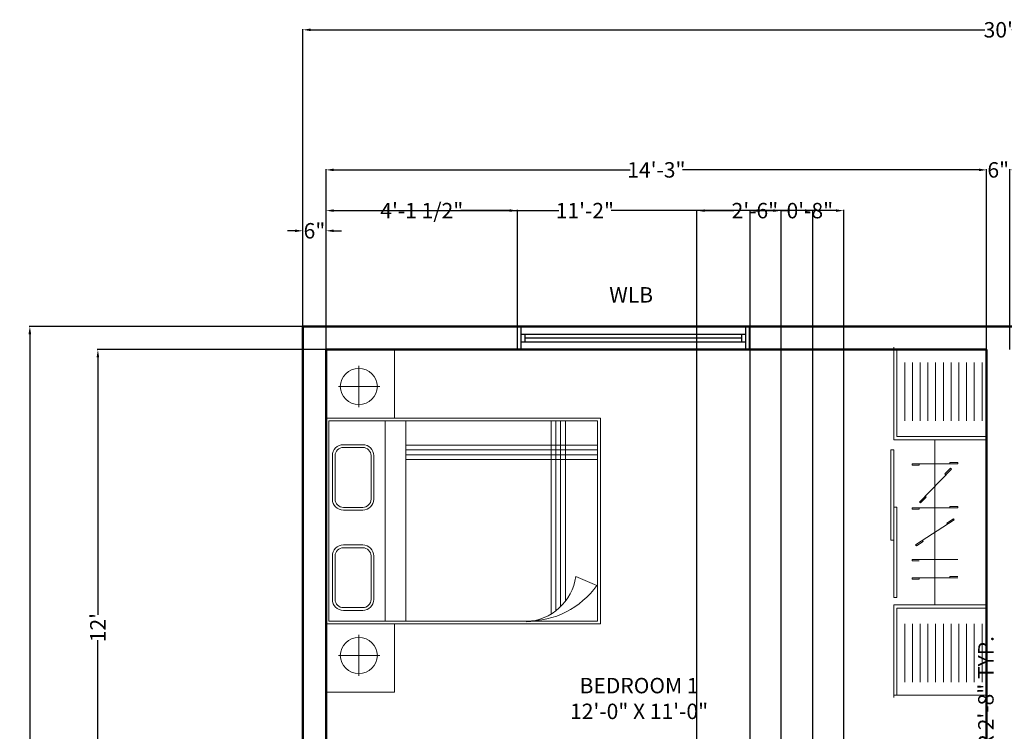
# Model space of a CAD drawing. Units: inches. Extents: x 2663 to 3147, y 140 to 736.
# Tile 5 of 6: x 2663 to 2918, y 551 to 736. Entities that reach past the tile are written whole.
import ezdxf

# ---------------------------------------------------------------- set-up
doc = ezdxf.new("R2010")
doc.units = ezdxf.units.IN
doc.header["$MEASUREMENT"] = 0
for name, color, linetype, lineweight in [('A-ANNO-DIMS', 2, 'Continuous', 18), ('A-AREA-IDEN', 3, 'Continuous', 25), ('A-FURN', 8, 'Continuous', 18), ('A-GLAZ', 4, 'Continuous', 25), ('A-WALL', 7, 'Continuous', 50)]:
    doc.layers.add(name, color=color, linetype=linetype, lineweight=lineweight)
doc.styles.get("Standard").update_dxf_attribs({"font": 'arial.ttf'})
doc.dimstyles.get("Standard").update_dxf_attribs({"dimtxt": 4, "dimasz": 2, "dimexe": 0.18, "dimexo": 0.0625, "dimgap": 0.09, "dimtad": 0, "dimdec": 0, "dimzin": 0, "dimdsep": 46, "dimlunit": 4, "dimtxsty": 'Standard', "dimcen": 0.09, "dimadec": 0, "dimazin": 0, "dimtfac": 1, "dimtdec": 0, "dimtofl": 0, "dimtmove": 0, "dimatfit": 3, "dimfxl": 1, "dimtolj": 1, "dimtzin": 0, "dimarcsym": 0})

# ---------------------------------------------------------------- blocks, each defined once
blk = doc.blocks.new('*D1')
at = {"layer": 'A-ANNO-DIMS', "color": 0, "lineweight": -2, "transparency": 16777216}
for p, q in [((2742.16, 650.39), (2742.16, 697.05)), ((2744.16, 696.87), (2820.89, 696.87)), ((2911.16, 696.87), (2834.43, 696.87)), ((2913.16, 650.39), (2913.16, 697.05))]:
    blk.add_line(p, q, dxfattribs=at)
at = {"layer": 'A-ANNO-DIMS', "color": 0, "transparency": 16777216}
for points in [[(2744.16, 697.21), (2744.16, 696.54), (2742.16, 696.87)], [(2911.16, 697.21), (2911.16, 696.54), (2913.16, 696.87)]]:
    blk.add_solid(points, dxfattribs=at)
at = {"layer": 'Defpoints', "color": 0, "transparency": 16777216}
for p in [(2913.16, 696.87), (2742.16, 650.32), (2913.16, 650.32)]:
    blk.add_point(p, dxfattribs=at)
at = {"layer": 'A-ANNO-DIMS', "color": 0, "transparency": 16777216, "insert": (2827.66, 696.87), "char_height": 4, "attachment_point": 5}
blk.add_mtext('\\A1;14\'-3"', dxfattribs=at)
blk = doc.blocks.new('*D2')
at = {"layer": 'A-ANNO-DIMS', "color": 0, "lineweight": -2, "transparency": 16777216}
for p, q in [((2911.16, 696.87), (2909.16, 696.87)), ((2913.16, 650.39), (2913.16, 697.05)), ((2919.16, 650.39), (2919.16, 697.05)), ((2921.16, 696.87), (2923.16, 696.87))]:
    blk.add_line(p, q, dxfattribs=at)
at = {"layer": 'A-ANNO-DIMS', "color": 0, "transparency": 16777216}
for points in [[(2911.16, 697.21), (2911.16, 696.54), (2913.16, 696.87)], [(2921.16, 697.21), (2921.16, 696.54), (2919.16, 696.87)]]:
    blk.add_solid(points, dxfattribs=at)
at = {"layer": 'Defpoints', "color": 0, "transparency": 16777216}
for p in [(2919.16, 696.87), (2913.16, 650.32), (2919.16, 650.32)]:
    blk.add_point(p, dxfattribs=at)
at = {"layer": 'A-ANNO-DIMS', "color": 0, "transparency": 16777216, "insert": (2916.16, 696.87), "char_height": 4, "attachment_point": 5}
blk.add_mtext('\\A1;6"', dxfattribs=at)
blk = doc.blocks.new('EDFRTYUI')
for p, q in [((3325.9, 253.54), (3325.9, 259.54)), ((3325.9, 259.54), (3385.9, 259.54)), ((3326.9, 253.54), (3326.9, 259.54)), ((3326.9, 257.54), (3384.9, 257.54)), ((3327.9, 255.54), (3327.9, 257.54)), ((3383.9, 257.54), (3383.9, 255.54)), ((3384.9, 259.54), (3384.9, 253.54)), ((3385.9, 259.54), (3385.9, 253.54)), ((3326.9, 255.54), (3384.9, 255.54)), ((3327.9, 256.54), (3383.9, 256.54)), ((3385.9, 253.54), (3325.9, 253.54))]:
    blk.add_line(p, q)
at = {"insert": (3337.87, 269.72), "char_height": 4, "attachment_point": 1}
blk.add_mtext_dynamic_manual_height_columns('\\pxqc;WLB', width=34.9199, gutter_width=20, heights=[0], dxfattribs=at)
blk = doc.blocks.new('A$C34930FF8')
at = {"ltscale": 0.05}
for p, q in [((0, 2252.4), (0, 16.8)), ((600, 2252.4), (0, 2252.4)), ((185.4, 1513), (185.4, 1521.5)), ((227.1, 1479.2), (233.2, 1485.2)), ((237.7, 1513), (237.7, 1521.5)), ((436.7, 1513), (436.7, 1504.4)), ((482.5, 1513), (482.5, 1504.4)), ((263.6, 1441.7), (269.7, 1447.7)), ((398.2, 1303.6), (392.1, 1297.6)), ((185.4, 1229.1), (185.4, 1237.7)), ((237.7, 1229.1), (237.7, 1237.7)), ((434.8, 1266.1), (428.7, 1260.1)), ((436.7, 1228.2), (436.7, 1219.7)), ((482.5, 1228.2), (482.5, 1219.7)), ((209.5, 1150.1), (214.1, 1157.3)), ((253.5, 1121.8), (258.1, 1129)), ((415.3, 1017.6), (410.6, 1010.5)), ((459.3, 989.3), (454.7, 982.1)), ((482.5, 894.9), (482.5, 886.3)), ((237.7, 775.3), (237.7, 783.9)), ((436.7, 775.3), (436.7, 766.8)), ((482.5, 775.3), (482.5, 766.8)), ((600, 16.8), (0, 16.8))]:
    blk.add_line(p, q, dxfattribs=at)
for p, q in [((580, 1690.9), (580, 2252.4)), ((600, 1669.3), (600, 2269.3)), ((30, 1790.9), (30, 2169.3)), ((80, 1790.9), (80, 2169.3)), ((130, 1790.9), (130, 2169.3)), ((180, 1790.9), (180, 2169.3)), ((230, 1790.9), (230, 2169.3)), ((280, 1790.9), (280, 2169.3)), ((330, 1790.9), (330, 2169.3)), ((380, 1790.9), (380, 2169.3)), ((430, 1790.9), (430, 2169.3)), ((480, 1790.9), (480, 2169.3)), ((530, 1790.9), (530, 2169.3)), ((580, 1690.9), (0, 1690.9)), ((600, 1669.3), (0, 1669.3)), ((335.4, 1666.1), (335.4, 603.1)), ((600, 1603.3), (620, 1603.3)), ((600, 1018.7), (600, 1603.3)), ((620, 1603.3), (620, 1018.7)), ((237.7, 1521.5), (185.4, 1521.5)), ((482.5, 1513), (185.4, 1513)), ((434.8, 1266.1), (227.4, 1478.9)), ((269.7, 1447.7), (233.2, 1485.2)), ((436.7, 1504.4), (482.5, 1504.4)), ((428.7, 1260.1), (392.1, 1297.6)), ((237.7, 1237.7), (185.4, 1237.7)), ((482.5, 1228.2), (185.4, 1228.2)), ((436.7, 1219.7), (482.5, 1219.7)), ((600, 1233.4), (580, 1233.4)), ((580, 1233.4), (580, 648.7)), ((600, 648.7), (600, 1233.4)), ((459.3, 989.3), (209.5, 1150.1)), ((258.1, 1129), (214.1, 1157.3)), ((454.7, 982.1), (410.6, 1010.5)), ((620, 1018.7), (600, 1018.7)), ((482.5, 894.9), (185.4, 894.9)), ((436.7, 886.3), (482.5, 886.3)), ((237.7, 783.9), (185.4, 783.9)), ((482.5, 775.3), (185.4, 775.3)), ((436.7, 766.8), (482.5, 766.8)), ((580, 648.7), (600, 648.7)), ((600, 600), (0, 600)), ((580, 578.3), (0, 578.3)), ((580, 578.3), (580, 16.8)), ((600, 600), (600, 0)), ((30, 478.3), (30, 100)), ((80, 478.3), (80, 100)), ((130, 478.3), (130, 100)), ((180, 478.3), (180, 100)), ((230, 478.3), (230, 100)), ((280, 478.3), (280, 100)), ((330, 478.3), (330, 100)), ((380, 478.3), (380, 100)), ((430, 478.3), (430, 100)), ((480, 478.3), (480, 100)), ((530, 478.3), (530, 100))]:
    blk.add_line(p, q)
blk = doc.blocks.new('A$C057D194F')
for p, q in [((0, 1.5, -0.1688), (0, 2, -0.1688)), ((0, 2, -0.1688), (0.5, 2, -0.1688)), ((0.5, 2, -0.1688), (0.5, 0, -0.1688)), ((2, 2, -0.1688), (0.5, 2, -0.1688)), ((1.98, 1.98, -0.1688), (0.52, 1.98, -0.1688)), ((0.52, 1.98, -0.1688), (0.52, 0.02, -0.1688)), ((1.0907, 1.9539, -0.1688), (0.7735, 1.9539, -0.1688)), ((1.8224, 1.9539, -0.1688), (1.5052, 1.9539, -0.1688)), ((1.98, 0.02, -0.1688), (1.98, 1.98, -0.1688)), ((2, 0, -0.1688), (2, 2, -0.1688)), ((2.5, 2, -0.1688), (2, 2, -0.1688)), ((2.5, 1.5, -0.1688), (2.5, 2, -0.1688)), ((0.2687, 1.9081, -0.1688), (0.2687, 1.761, -0.1688)), ((0.2687, 1.6081, -0.1688), (0.2687, 1.9081, -0.1688)), ((0.6935, 1.8739, -0.1688), (0.6935, 1.7322, -0.1688)), ((0.7135, 1.8739, -0.1688), (0.7135, 1.7322, -0.1688)), ((1.0907, 1.9339, -0.1688), (0.7735, 1.9339, -0.1688)), ((1.1507, 1.7322, -0.1688), (1.1507, 1.8739, -0.1688)), ((1.1707, 1.7322, -0.1688), (1.1707, 1.8739, -0.1688)), ((1.4252, 1.8739, -0.1688), (1.4252, 1.7322, -0.1688)), ((1.4452, 1.8739, -0.1688), (1.4452, 1.7322, -0.1688)), ((1.8224, 1.9339, -0.1688), (1.5052, 1.9339, -0.1688)), ((1.8824, 1.7322, -0.1688), (1.8824, 1.8739, -0.1688)), ((1.9024, 1.7322, -0.1688), (1.9024, 1.8739, -0.1688)), ((2.2313, 1.9081, -0.1688), (2.2313, 1.761, -0.1688)), ((2.2313, 1.6081, -0.1688), (2.2313, 1.9081, -0.1688)), ((0.4194, 1.761, -0.1688), (0.1194, 1.761, -0.1688)), ((0.2687, 1.761, -0.1688), (0.4194, 1.761, -0.1688)), ((0.2687, 1.761, -0.1688), (0.2687, 1.6081, -0.1688)), ((2.0806, 1.761, -0.1688), (2.3806, 1.761, -0.1688)), ((2.2313, 1.761, -0.1688), (2.0806, 1.761, -0.1688)), ((2.2313, 1.761, -0.1688), (2.2313, 1.6081, -0.1688)), ((0.7735, 1.6722, -0.1688), (1.0907, 1.6722, -0.1688)), ((0.7735, 1.6522, -0.1688), (1.0907, 1.6522, -0.1688)), ((1.5052, 1.6722, -0.1688), (1.8224, 1.6722, -0.1688)), ((1.5052, 1.6522, -0.1688), (1.8224, 1.6522, -0.1688)), ((1.98, 1.5693, -0.1688), (0.52, 1.5693, -0.1688)), ((0.5, 1.5, -0.1688), (0, 1.5, -0.1688)), ((2, 1.5, -0.1688), (2.5, 1.5, -0.1688)), ((1.98, 1.4193, -0.1688), (0.52, 1.4193, -0.1688)), ((0.6969, 0.02, -0.1688), (0.6969, 1.4193, -0.1688)), ((0.7319, 0.02, -0.1688), (0.7319, 1.4193, -0.1688)), ((0.7669, 0.02, -0.1688), (0.7669, 1.4193, -0.1688)), ((0.8019, 0.02, -0.1688), (0.8019, 1.4193, -0.1688)), ((0.52, 0.3595, -0.1688), (1.9292, 0.3595, -0.1688)), ((0.52, 0.3245, -0.1688), (1.905, 0.3245, -0.1688)), ((0.52, 0.2895, -0.1688), (1.8742, 0.2895, -0.1688)), ((0.52, 0.2545, -0.1688), (1.8344, 0.2545, -0.1688)), ((1.6548, 0.1789, -0.1688), (1.7198, 0.0251, -0.1688)), ((0.52, 0.02, -0.1688), (1.98, 0.02, -0.1688)), ((0.5, 0, -0.1688), (2, 0, -0.1688))]:
    blk.add_line(p, q)
for centre, radius, start, end in [((0.7735, 1.8739, -0.1688), 0.08, 90, 180), ((1.0907, 1.8739, -0.1688), 0.08, 0, 90), ((1.5052, 1.8739, -0.1688), 0.08, 90, 180), ((1.8224, 1.8739, -0.1688), 0.08, 0, 90), ((0.7735, 1.8739, -0.1688), 0.06, 90, 180), ((1.0907, 1.8739, -0.1688), 0.06, 0, 90), ((1.5052, 1.8739, -0.1688), 0.06, 90, 180), ((1.8224, 1.8739, -0.1688), 0.06, 0, 90), ((0.7735, 1.7322, -0.1688), 0.08, 180, 270), ((0.7735, 1.7322, -0.1688), 0.06, 180, 270), ((1.0907, 1.7322, -0.1688), 0.08, 270, 0), ((1.0907, 1.7322, -0.1688), 0.06, 270, 0), ((1.5052, 1.7322, -0.1688), 0.08, 180, 270), ((1.5052, 1.7322, -0.1688), 0.06, 180, 270), ((1.8224, 1.7322, -0.1688), 0.08, 270, 0), ((1.8224, 1.7322, -0.1688), 0.06, 270, 0), ((1.5992, 0.5623, -0.1688), 0.3874, 278.2518, 356.6808), ((1.363, 0.5286, -0.1688), 0.6171, 305.32946, 1.04595)]:
    blk.add_arc(centre, radius, start, end)
blk.add_ellipse((0.2687, 1.761, -0.1688), major_axis=(0, -0.1351), ratio=0.975448)
at = {"extrusion": (0, 0, -1)}
blk.add_ellipse((2.2313, 1.761, -0.1688), major_axis=(0, 0.1351), ratio=0.975448, dxfattribs=at)
for p in [(0.2687, 1.761, -0.1688), (2.2313, 1.761, -0.1688)]:
    blk.add_point(p)
blk = doc.blocks.new('*D21')
at = {"layer": 'A-ANNO-DIMS', "color": 0, "lineweight": -2, "transparency": 16777216}
for p, q in [((2734.16, 681.1), (2732.16, 681.1)), ((2736.16, 656.39), (2736.16, 681.28)), ((2742.16, 650.39), (2742.16, 681.28)), ((2744.16, 681.1), (2746.16, 681.1))]:
    blk.add_line(p, q, dxfattribs=at)
at = {"layer": 'A-ANNO-DIMS', "color": 0, "transparency": 16777216}
for points in [[(2734.16, 681.43), (2734.16, 680.76), (2736.16, 681.1)], [(2744.16, 681.43), (2744.16, 680.76), (2742.16, 681.1)]]:
    blk.add_solid(points, dxfattribs=at)
at = {"layer": 'Defpoints', "color": 0, "transparency": 16777216}
for p in [(2742.16, 681.1), (2736.16, 656.32), (2742.16, 650.32)]:
    blk.add_point(p, dxfattribs=at)
at = {"layer": 'A-ANNO-DIMS', "color": 0, "transparency": 16777216, "insert": (2739.16, 681.1), "char_height": 4, "attachment_point": 5}
blk.add_mtext('\\A1;6"', dxfattribs=at)
blk = doc.blocks.new('*D36')
at = {"layer": 'A-ANNO-DIMS', "color": 0, "lineweight": -2, "transparency": 16777216}
for p, q in [((2742.1, 650.32), (2682.92, 650.32)), ((2683.1, 648.32), (2683.1, 581.62)), ((2683.1, 508.32), (2683.1, 575.03)), ((2742.1, 506.32), (2682.92, 506.32))]:
    blk.add_line(p, q, dxfattribs=at)
at = {"layer": 'A-ANNO-DIMS', "color": 0, "transparency": 16777216}
for points in [[(2682.77, 648.32), (2683.44, 648.32), (2683.1, 650.32)], [(2682.77, 508.32), (2683.44, 508.32), (2683.1, 506.32)]]:
    blk.add_solid(points, dxfattribs=at)
at = {"layer": 'Defpoints', "color": 0, "transparency": 16777216}
for p in [(2683.1, 650.32), (2742.16, 650.32), (2742.16, 506.32)]:
    blk.add_point(p, dxfattribs=at)
at = {"layer": 'A-ANNO-DIMS', "color": 0, "transparency": 16777216, "insert": (2683.1, 578.32), "char_height": 4, "attachment_point": 5, "rotation": 90}
blk.add_mtext("\\A1;12'", dxfattribs=at)
blk = doc.blocks.new('*D37')
at = {"layer": 'A-ANNO-DIMS', "color": 0, "lineweight": -2, "transparency": 16777216}
for p, q in [((2736.1, 656.32), (2665.31, 656.32)), ((2665.49, 654.32), (2665.49, 419.89)), ((2665.49, 178.32), (2665.49, 412.76)), ((2736.1, 176.32), (2665.31, 176.32))]:
    blk.add_line(p, q, dxfattribs=at)
at = {"layer": 'A-ANNO-DIMS', "color": 0, "transparency": 16777216}
for points in [[(2665.15, 654.32), (2665.82, 654.32), (2665.49, 656.32)], [(2665.15, 178.32), (2665.82, 178.32), (2665.49, 176.32)]]:
    blk.add_solid(points, dxfattribs=at)
at = {"layer": 'Defpoints', "color": 0, "transparency": 16777216}
for p in [(2665.49, 656.32), (2736.16, 656.32), (2736.16, 176.32)]:
    blk.add_point(p, dxfattribs=at)
at = {"layer": 'A-ANNO-DIMS', "color": 0, "transparency": 16777216, "insert": (2665.49, 416.32), "char_height": 4, "attachment_point": 5, "rotation": 90}
blk.add_mtext("\\A1;40'", dxfattribs=at)
blk = doc.blocks.new('*D38')
at = {"layer": 'A-ANNO-DIMS', "color": 0, "lineweight": -2, "transparency": 16777216}
for p, q in [((2736.16, 656.39), (2736.16, 733.33)), ((2738.16, 733.15), (2912.68, 733.15)), ((3094.16, 733.15), (2919.64, 733.15)), ((3096.16, 656.39), (3096.16, 733.33))]:
    blk.add_line(p, q, dxfattribs=at)
at = {"layer": 'A-ANNO-DIMS', "color": 0, "transparency": 16777216}
for points in [[(2738.16, 733.48), (2738.16, 732.82), (2736.16, 733.15)], [(3094.16, 733.48), (3094.16, 732.82), (3096.16, 733.15)]]:
    blk.add_solid(points, dxfattribs=at)
at = {"layer": 'Defpoints', "color": 0, "transparency": 16777216}
for p in [(3096.16, 733.15), (2736.16, 656.32), (3096.16, 656.32)]:
    blk.add_point(p, dxfattribs=at)
at = {"layer": 'A-ANNO-DIMS', "color": 0, "transparency": 16777216, "insert": (2916.16, 733.15), "char_height": 4, "attachment_point": 5}
blk.add_mtext("\\A1;30'", dxfattribs=at)
blk = doc.blocks.new('*D39')
at = {"layer": 'A-ANNO-DIMS', "color": 0, "lineweight": -2, "transparency": 16777216}
for p, q in [((2912.96, 532.32), (2912.96, 534.32)), ((2908.22, 532.32), (2913.14, 532.32)), ((2912.96, 502.32), (2912.96, 530.32)), ((2908.22, 500.32), (2913.14, 500.32))]:
    blk.add_line(p, q, dxfattribs=at)
at = {"layer": 'A-ANNO-DIMS', "color": 0, "transparency": 16777216}
for points in [[(2912.63, 530.32), (2913.29, 530.32), (2912.96, 532.32)], [(2912.63, 502.32), (2913.29, 502.32), (2912.96, 500.32)]]:
    blk.add_solid(points, dxfattribs=at)
at = {"layer": 'Defpoints', "color": 0, "transparency": 16777216}
for p in [(2908.16, 532.32), (2912.96, 532.32), (2908.16, 500.32)]:
    blk.add_point(p, dxfattribs=at)
at = {"layer": 'A-ANNO-DIMS', "color": 0, "transparency": 16777216, "insert": (2912.96, 555.66), "char_height": 4, "attachment_point": 5, "rotation": 90}
blk.add_mtext('\\A1;DOOR 2\'-8" TYP.', dxfattribs=at)
blk = doc.blocks.new('*D61')
at = {"layer": 'A-ANNO-DIMS', "color": 0, "lineweight": -2, "transparency": 16777216}
for p, q in [((2851.95, 276.84), (2851.95, 686.5)), ((2853.95, 686.32), (2857.98, 686.32)), ((2859.98, 276.84), (2859.98, 686.5)), ((2859.98, 686.32), (2861.98, 686.32))]:
    blk.add_line(p, q, dxfattribs=at)
at = {"layer": 'A-ANNO-DIMS', "color": 0, "transparency": 16777216}
for points in [[(2853.95, 686.66), (2853.95, 685.99), (2851.95, 686.32)], [(2857.98, 686.66), (2857.98, 685.99), (2859.98, 686.32)]]:
    blk.add_solid(points, dxfattribs=at)
at = {"layer": 'Defpoints', "color": 0, "transparency": 16777216}
for p in [(2859.98, 686.32), (2851.95, 276.78), (2859.98, 276.78)]:
    blk.add_point(p, dxfattribs=at)
at = {"layer": 'A-ANNO-DIMS', "color": 0, "transparency": 16777216, "insert": (2867.39, 686.32), "char_height": 4, "attachment_point": 5}
blk.add_mtext('\\A1;0\'-8"', dxfattribs=at)
blk = doc.blocks.new('*D68')
at = {"layer": 'A-ANNO-DIMS', "color": 0, "lineweight": -2, "transparency": 16777216}
for p, q in [((2742.16, 650.39), (2742.16, 686.5)), ((2744.16, 686.32), (2756.79, 686.32)), ((2789.71, 686.32), (2777.08, 686.32)), ((2791.71, 650.39), (2791.71, 686.5))]:
    blk.add_line(p, q, dxfattribs=at)
at = {"layer": 'A-ANNO-DIMS', "color": 0, "transparency": 16777216}
for points in [[(2744.16, 686.66), (2744.16, 685.99), (2742.16, 686.32)], [(2789.71, 686.66), (2789.71, 685.99), (2791.71, 686.32)]]:
    blk.add_solid(points, dxfattribs=at)
at = {"layer": 'Defpoints', "color": 0, "transparency": 16777216}
for p in [(2791.71, 686.32), (2742.16, 650.32), (2791.71, 650.32)]:
    blk.add_point(p, dxfattribs=at)
at = {"layer": 'A-ANNO-DIMS', "color": 0, "transparency": 16777216, "insert": (2766.94, 686.32), "char_height": 4, "attachment_point": 5}
blk.add_mtext('\\A1;4\'-1 1/2"', dxfattribs=at)
blk = doc.blocks.new('*D75')
at = {"layer": 'A-ANNO-DIMS', "color": 0, "lineweight": -2, "transparency": 16777216}
for p, q in [((2742.16, 506.39), (2742.16, 686.5)), ((2744.16, 686.32), (2802.39, 686.32)), ((2874.16, 686.32), (2815.93, 686.32)), ((2876.16, 506.39), (2876.16, 686.5))]:
    blk.add_line(p, q, dxfattribs=at)
at = {"layer": 'A-ANNO-DIMS', "color": 0, "transparency": 16777216}
for points in [[(2744.16, 686.66), (2744.16, 685.99), (2742.16, 686.32)], [(2874.16, 686.66), (2874.16, 685.99), (2876.16, 686.32)]]:
    blk.add_solid(points, dxfattribs=at)
at = {"layer": 'Defpoints', "color": 0, "transparency": 16777216}
for p in [(2876.16, 686.32), (2742.16, 506.32), (2876.16, 506.32)]:
    blk.add_point(p, dxfattribs=at)
at = {"layer": 'A-ANNO-DIMS', "color": 0, "transparency": 16777216, "insert": (2809.16, 686.32), "char_height": 4, "attachment_point": 5}
blk.add_mtext('\\A1;11\'-2"', dxfattribs=at)
blk = doc.blocks.new('*D78')
at = {"layer": 'A-ANNO-DIMS', "color": 0, "lineweight": -2, "transparency": 16777216}
for p, q in [((2838.16, 440.39), (2838.16, 686.5)), ((2840.16, 686.32), (2847.72, 686.32)), ((2866.16, 686.32), (2858.6, 686.32)), ((2868.16, 440.39), (2868.16, 686.5))]:
    blk.add_line(p, q, dxfattribs=at)
at = {"layer": 'A-ANNO-DIMS', "color": 0, "transparency": 16777216}
for points in [[(2840.16, 686.66), (2840.16, 685.99), (2838.16, 686.32)], [(2866.16, 686.66), (2866.16, 685.99), (2868.16, 686.32)]]:
    blk.add_solid(points, dxfattribs=at)
at = {"layer": 'Defpoints', "color": 0, "transparency": 16777216}
for p in [(2868.16, 686.32), (2838.16, 440.32), (2868.16, 440.32)]:
    blk.add_point(p, dxfattribs=at)
at = {"layer": 'A-ANNO-DIMS', "color": 0, "transparency": 16777216, "insert": (2853.16, 686.32), "char_height": 4, "attachment_point": 5}
blk.add_mtext('\\A1;2\'-6"', dxfattribs=at)

msp = doc.modelspace()

# ---------------------------------------------------------------- linework, layer by layer
at = {"layer": 'A-WALL'}
for p, q in [((2736.16, 656.32), (3096.16, 656.32)), ((2736.16, 176.32), (2736.16, 656.32)), ((2742.16, 650.32), (2913.16, 650.32)), ((2742.16, 506.32), (2742.16, 650.32)), ((2913.16, 650.32), (2913.16, 506.32))]:
    msp.add_line(p, q, dxfattribs=at)

# ---------------------------------------------------------------- block references
at = {"layer": 'A-FURN', "xscale": -35.50398587953096, "yscale": 35.50398587953096, "zscale": 35.50398587953096, "rotation": 90}
msp.add_blockref('A$C057D194F', (2813.17, 650.32, 5.99), dxfattribs=at)
at = {"layer": 'A-FURN', "xscale": -0.0400188077054237, "yscale": 0.0400188077054237, "zscale": 0.0400188077054237}
msp.add_blockref('A$C34930FF8', (2913.16, 560.18), dxfattribs=at)
at = {"layer": 'A-GLAZ'}
msp.add_blockref('EDFRTYUI', (-534.19, 396.79), dxfattribs=at)

# ---------------------------------------------------------------- texts
at = {"layer": 'A-AREA-IDEN', "insert": (2782.38, 565.3), "char_height": 4, "attachment_point": 1}
msp.add_mtext_dynamic_manual_height_columns('\\pxqc;BEDROOM 1\\P12\'-0" X 11\'-0"', width=81.6207, gutter_width=20, heights=[0], dxfattribs=at)

# ---------------------------------------------------------------- dimensions: what is measured, and where the dimension line sits
at = {"layer": 'A-ANNO-DIMS'}
for base, p1, p2, override, picture, middle in [((3096.16, 733.15), (2736.16, 656.32), (3096.16, 656.32), {"dimclrd": 0, "dimclre": 0, "dimclrt": 0}, '*D38', (2916.16, 733.15)), ((2913.16, 696.87), (2742.16, 650.32), (2913.16, 650.32), {"dimclrd": 0, "dimclre": 0, "dimclrt": 0}, '*D1', (2827.66, 696.87)), ((2919.16, 696.87), (2913.16, 650.32), (2919.16, 650.32), {"dimclrd": 0, "dimclre": 0, "dimclrt": 0}, '*D2', (2916.16, 696.87)), ((2791.7116, 686.3237), (2742.1615, 650.3237), (2791.7116, 650.3237), {"dimdec": 1, "dimlfac": 1, "dimrnd": 0, "dimzin": 1, "dimdsep": 46, "dimlunit": 4, "dimfrac": 2}, '*D68', (2766.9365, 686.3237)), ((2876.16, 686.32), (2742.16, 506.32), (2876.16, 506.32), {"dimdec": 1, "dimlfac": 1, "dimrnd": 0, "dimzin": 1, "dimdsep": 46, "dimlunit": 4, "dimfrac": 2}, '*D75', (2809.16, 686.32)), ((2868.16, 686.32), (2838.16, 440.32), (2868.16, 440.32), {"dimdec": 1, "dimlfac": 1, "dimrnd": 0, "dimzin": 1, "dimdsep": 46, "dimlunit": 4, "dimfrac": 2}, '*D78', (2853.16, 686.32)), ((2859.98, 686.32), (2851.95, 276.78), (2859.98, 276.78), {"dimdec": 1, "dimlfac": 1, "dimrnd": 0, "dimzin": 1, "dimdsep": 46, "dimlunit": 4, "dimfrac": 2}, '*D61', (2867.39, 686.32)), ((2742.16, 681.1), (2736.16, 656.32), (2742.16, 650.32), {"dimclrd": 0, "dimclre": 0, "dimclrt": 0}, '*D21', (2739.16, 681.1))]:
    dim = msp.add_linear_dim(base=base, p1=p1, p2=p2, dimstyle='Standard', override=override, dxfattribs=at)
    dim.commit()
    dim.dimension.update_dxf_attribs({"geometry": picture, "text_midpoint": middle})
for base, p1, p2, picture, middle in [((2665.49, 656.32), (2736.16, 176.32), (2736.16, 656.32), '*D37', (2665.49, 416.32)), ((2683.1, 650.32), (2742.16, 506.32), (2742.16, 650.32), '*D36', (2683.1, 578.32))]:
    dim = msp.add_linear_dim(base=base, p1=p1, p2=p2, angle=90, dimstyle='Standard', override={"dimclrd": 0, "dimclre": 0, "dimclrt": 0}, dxfattribs=at)
    dim.commit()
    dim.dimension.update_dxf_attribs({"geometry": picture, "text_midpoint": middle})
dim = msp.add_linear_dim(base=(2912.96, 532.32), p1=(2908.16, 500.32), p2=(2908.16, 532.32), angle=90, text='DOOR <> TYP.', dimstyle='Standard', override={"dimdec": 1, "dimrnd": 0, "dimzin": 1, "dimlunit": 4, "dimfrac": 2}, dxfattribs=at)
dim.commit()
dim.dimension.update_dxf_attribs({"geometry": '*D39', "text_midpoint": (2912.96, 555.66)})

doc.saveas('drawing.dxf')
